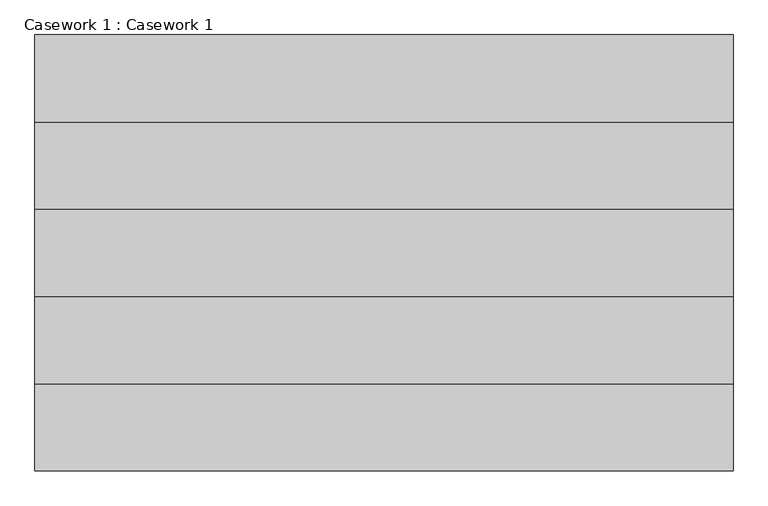
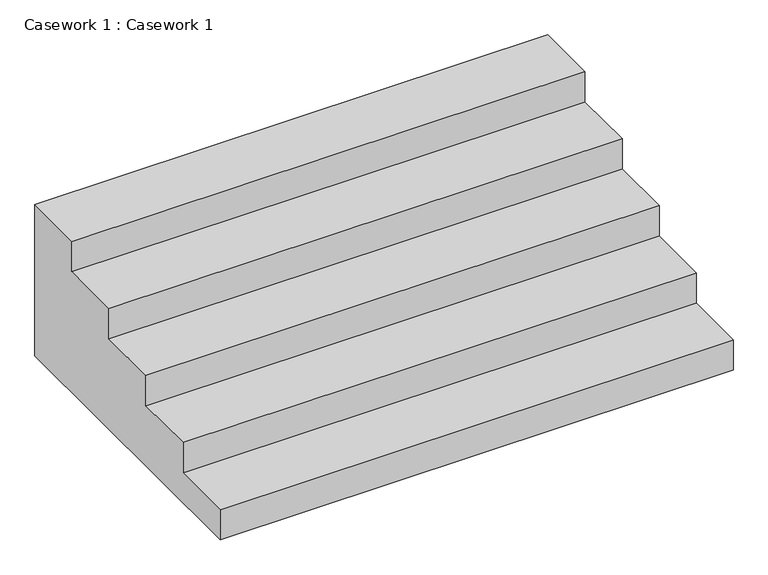
"""IFC4 building model written with IfcOpenShell, lengths in millimetres: furniture geometry, Casework 1 : Casework 1."""

from ifc_helpers import new_model, si_unit, frame, origin, place, context, project, spatial, polyline, outline, extrude, source, transform, mapped, element, save


def casework_1_casework_1_a8a15752(model_context):
    return source(origin(), model_context, "Body", "SweptSolid", [
        extrude(outline(polyline([(-172.3093114, 762.0), (132.4906886, 762.0), (132.4906886, 0.0), (-1391.5093114, 0.0), (-1391.5093114, 152.4), (-1086.7093114, 152.4), (-1086.7093114, 304.8), (-781.9093114, 304.8), (-781.9093114, 457.2), (-477.1093114, 457.2), (-477.1093114, 609.6), (-172.3093114, 609.6), (-172.3093114, 762.0)])), frame((3712.0512825, 0.0, 0.0), z_axis=(1.0, 0.0, 0.0), x_axis=(0.0, 1.0, 0.0)), (0.0, 0.0, 1.0), 2438.4),
    ])


if __name__ == "__main__":
    model = new_model("IFC4")
    model_context = context("Model", 3, world=origin())
    ifc_project = project(units=[si_unit("LENGTHUNIT", "METRE", prefix="MILLI")], contexts=[model_context])
    site = spatial("IfcSite", under=ifc_project)
    building = spatial("IfcBuilding", under=site)
    placement = place(None, origin())
    casework_1_casework_1_shape = casework_1_casework_1_a8a15752(model_context)
    element("IfcFurniture", 1, ObjectType="Casework 1 : Casework 1", at=placement, inside=building, context=model_context, shape_type="MappedRepresentation", body=[
        mapped(casework_1_casework_1_shape, transform((0.0, 0.0, 0.0), x_axis=(1.0, 0.0, 0.0), y_axis=(0.0, 1.0, 0.0), z_axis=(0.0, 0.0, 1.0))),
    ])
    save(model, "model.ifc")

# Revit data of these elements
# Element 1 (IfcFurniture, "Casework 1 : Casework 1")
#   Materials on its faces: "Black, Glossy"
# Materials
#   "Black, Glossy": colour RGB 128 128 128, transparency 0
